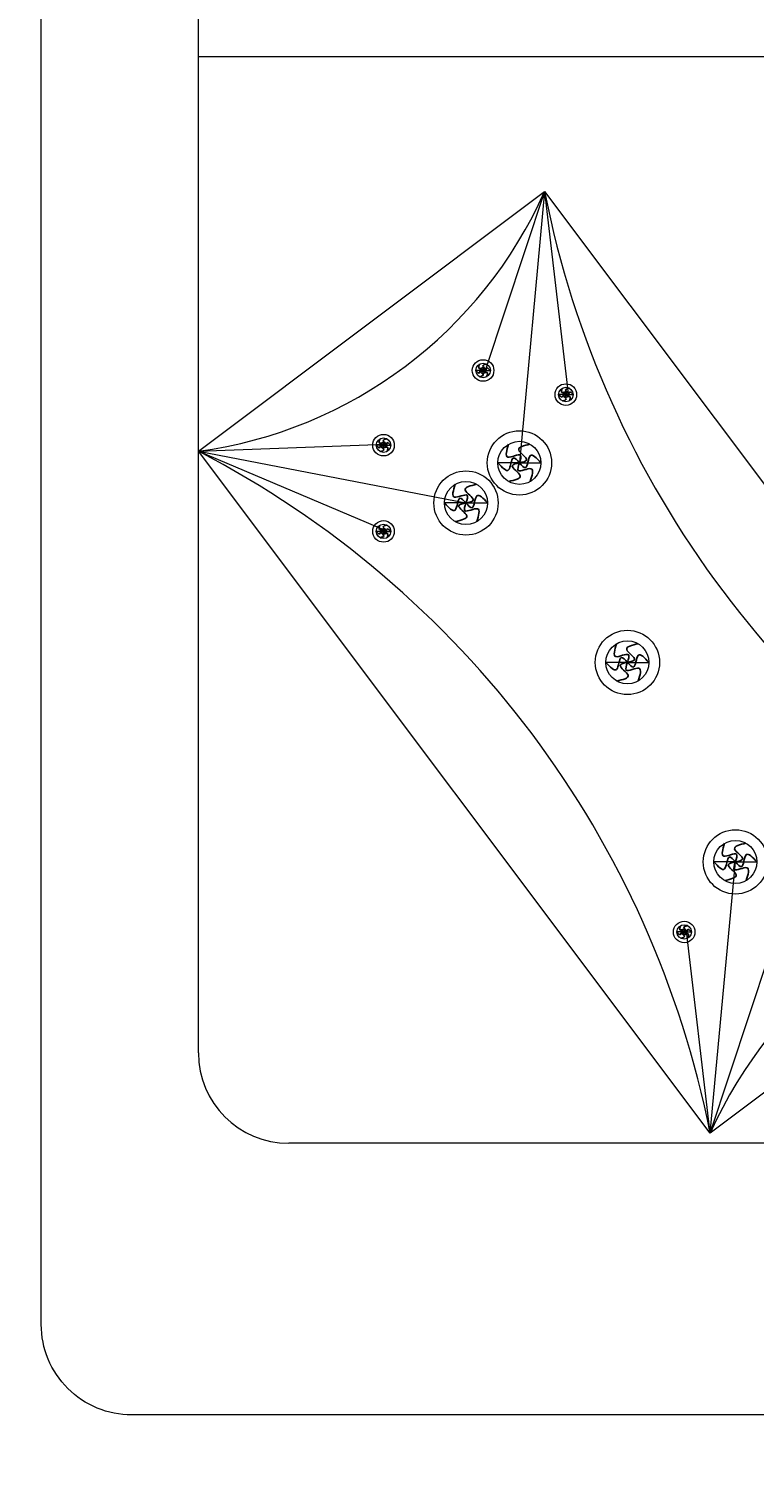
# Model space of a CAD drawing. Units: inches. Extents: x -61 to 1599, y -1316 to 257.
# Tile 102 of 204: x 126 to 142, y -131 to -99. Entities that reach past the tile are written whole.
import ezdxf

# ---------------------------------------------------------------- set-up
doc = ezdxf.new("R2010")
doc.units = ezdxf.units.IN
doc.header["$MEASUREMENT"] = 0
doc.layers.add('A-ANNO-DIMS', color=2, linetype='Continuous', lineweight=18)
doc.layers.add('FURNITURE', color=83, linetype='Continuous', lineweight=18)
doc.layers.add('FUR', color=83, linetype='Continuous')
doc.styles.get("Standard").update_dxf_attribs({"font": 'arial.ttf'})
doc.dimstyles.get("Standard").update_dxf_attribs({"dimtxt": 0.18, "dimasz": 0.18, "dimexe": 0.18, "dimexo": 0.0625, "dimgap": 0.09, "dimtad": 0, "dimtih": 1, "dimtoh": 1, "dimdec": 0, "dimzin": 0, "dimdsep": 46, "dimlunit": 3, "dimtxsty": 'Standard', "dimcen": 0.09, "dimadec": 0, "dimazin": 0, "dimtfac": 1, "dimtdec": 0, "dimtofl": 0, "dimtmove": 0, "dimatfit": 3, "dimfxl": 1, "dimtolj": 1, "dimtzin": 0, "dimarcsym": 0})

# ---------------------------------------------------------------- blocks, each defined once
blk = doc.blocks.new('*U160')
at = {"layer": 'FUR'}
blk.add_open_spline([(0.005, 0.08), (-0.03, 0.048), (-0.098, -0.015), (0.075, -0.018), (0.024, -0.063), (0.005, -0.08)], degree=3, knots=[0, 0, 0, 0, 0.0954578, 0.1898773, 0.2470677, 0.2470677, 0.2470677, 0.2470677], dxfattribs=at)
blk = doc.blocks.new('*U161')
at = {"layer": 'FUR', "transparency": 16777216}
for p, rotation in [((222.173, -79.977), 60), ((222.312, -79.968), 300), ((222.317, -80.048), 240), ((222.178, -80.056), 120), ((222.25, -80.092), 180)]:
    blk.add_blockref('*U160', p, dxfattribs=dict(at, rotation=rotation))
blk.add_blockref('*U160', (222.24, -79.932), dxfattribs=at)
blk = doc.blocks.new('*U172')
at = {"layer": 'FUR'}
blk.add_open_spline([(0.005, 0.08), (-0.03, 0.048), (-0.098, -0.015), (0.075, -0.018), (0.024, -0.063), (0.005, -0.08)], degree=3, knots=[0, 0, 0, 0, 0.0954578, 0.1898773, 0.2470677, 0.2470677, 0.2470677, 0.2470677], dxfattribs=at)
blk = doc.blocks.new('*U173')
at = {"layer": 'FUR', "transparency": 16777216}
for p, rotation in [((222.173, -79.977), 60), ((222.312, -79.968), 300), ((222.317, -80.048), 240), ((222.178, -80.056), 120), ((222.25, -80.092), 180)]:
    blk.add_blockref('*U172', p, dxfattribs=dict(at, rotation=rotation))
blk.add_blockref('*U172', (222.24, -79.932), dxfattribs=at)
blk = doc.blocks.new('*U184')
at = {"layer": 'FUR'}
blk.add_open_spline([(0.015, 0.238), (-0.088, 0.143), (-0.292, -0.045), (0.224, -0.053), (0.072, -0.187), (0.015, -0.238)], degree=3, knots=[0, 0, 0, 0, 0.2846533, 0.5662105, 0.736751, 0.736751, 0.736751, 0.736751], dxfattribs=at)
blk = doc.blocks.new('*U159')
at = {"layer": 'FUR', "transparency": 16777216}
for p, rotation in [((662.517, -238.489), 60), ((662.929, -238.463), 300), ((662.531, -238.727), 120), ((662.745, -238.833), 180), ((662.944, -238.702), 240)]:
    blk.add_blockref('*U184', p, dxfattribs=dict(at, rotation=rotation))
blk.add_blockref('*U184', (662.716, -238.357), dxfattribs=at)
blk = doc.blocks.new('*U174')
at = {"layer": 'FUR'}
blk.add_open_spline([(0.005, 0.08), (-0.03, 0.048), (-0.098, -0.015), (0.075, -0.018), (0.024, -0.063), (0.005, -0.08)], degree=3, knots=[0, 0, 0, 0, 0.0954578, 0.1898773, 0.2470677, 0.2470677, 0.2470677, 0.2470677], dxfattribs=at)
blk = doc.blocks.new('*U175')
at = {"layer": 'FUR', "transparency": 16777216}
for p, rotation in [((222.173, -79.977), 60), ((222.312, -79.968), 300), ((222.317, -80.048), 240), ((222.178, -80.056), 120), ((222.25, -80.092), 180)]:
    blk.add_blockref('*U174', p, dxfattribs=dict(at, rotation=rotation))
blk.add_blockref('*U174', (222.24, -79.932), dxfattribs=at)
blk = doc.blocks.new('*U168')
at = {"layer": 'FUR'}
blk.add_open_spline([(0.015, 0.238), (-0.088, 0.143), (-0.292, -0.045), (0.224, -0.053), (0.072, -0.187), (0.015, -0.238)], degree=3, knots=[0, 0, 0, 0, 0.2846533, 0.5662105, 0.736751, 0.736751, 0.736751, 0.736751], dxfattribs=at)
blk = doc.blocks.new('*U169')
at = {"layer": 'FUR', "transparency": 16777216}
for p, rotation in [((662.517, -238.489), 60), ((662.929, -238.463), 300), ((662.531, -238.727), 120), ((662.745, -238.833), 180), ((662.944, -238.702), 240)]:
    blk.add_blockref('*U168', p, dxfattribs=dict(at, rotation=rotation))
blk.add_blockref('*U168', (662.716, -238.357), dxfattribs=at)
blk = doc.blocks.new('*U176')
at = {"layer": 'FUR'}
blk.add_open_spline([(0.005, 0.08), (-0.03, 0.048), (-0.098, -0.015), (0.075, -0.018), (0.024, -0.063), (0.005, -0.08)], degree=3, knots=[0, 0, 0, 0, 0.0954578, 0.1898773, 0.2470677, 0.2470677, 0.2470677, 0.2470677], dxfattribs=at)
blk = doc.blocks.new('*U177')
at = {"layer": 'FUR', "transparency": 16777216}
for p, rotation in [((222.173, -79.977), 60), ((222.312, -79.968), 300), ((222.317, -80.048), 240), ((222.178, -80.056), 120), ((222.25, -80.092), 180)]:
    blk.add_blockref('*U176', p, dxfattribs=dict(at, rotation=rotation))
blk.add_blockref('*U176', (222.24, -79.932), dxfattribs=at)
blk = doc.blocks.new('*U170')
at = {"layer": 'FUR'}
blk.add_open_spline([(0.015, 0.238), (-0.088, 0.143), (-0.292, -0.045), (0.224, -0.053), (0.072, -0.187), (0.015, -0.238)], degree=3, knots=[0, 0, 0, 0, 0.2846533, 0.5662105, 0.736751, 0.736751, 0.736751, 0.736751], dxfattribs=at)
blk = doc.blocks.new('*U171')
at = {"layer": 'FUR', "transparency": 16777216}
for p, rotation in [((662.517, -238.489), 60), ((662.929, -238.463), 300), ((662.531, -238.727), 120), ((662.745, -238.833), 180), ((662.944, -238.702), 240)]:
    blk.add_blockref('*U170', p, dxfattribs=dict(at, rotation=rotation))
blk.add_blockref('*U170', (662.716, -238.357), dxfattribs=at)
blk = doc.blocks.new('*U164')
at = {"layer": 'FUR'}
blk.add_open_spline([(0.005, 0.08), (-0.03, 0.048), (-0.098, -0.015), (0.075, -0.018), (0.024, -0.063), (0.005, -0.08)], degree=3, knots=[0, 0, 0, 0, 0.0954578, 0.1898773, 0.2470677, 0.2470677, 0.2470677, 0.2470677], dxfattribs=at)
blk = doc.blocks.new('*U165')
at = {"layer": 'FUR', "transparency": 16777216}
for p, rotation in [((222.173, -79.977), 60), ((222.312, -79.968), 300), ((222.317, -80.048), 240), ((222.178, -80.056), 120), ((222.25, -80.092), 180)]:
    blk.add_blockref('*U164', p, dxfattribs=dict(at, rotation=rotation))
blk.add_blockref('*U164', (222.24, -79.932), dxfattribs=at)
blk = doc.blocks.new('*U183')
at = {"layer": 'FUR'}
blk.add_open_spline([(0.015, 0.238), (-0.088, 0.143), (-0.292, -0.045), (0.224, -0.053), (0.072, -0.187), (0.015, -0.238)], degree=3, knots=[0, 0, 0, 0, 0.2846533, 0.5662105, 0.736751, 0.736751, 0.736751, 0.736751], dxfattribs=at)
blk = doc.blocks.new('*U162')
at = {"layer": 'FUR', "transparency": 16777216}
for p, rotation in [((662.517, -238.489), 60), ((662.929, -238.463), 300), ((662.531, -238.727), 120), ((662.745, -238.833), 180), ((662.944, -238.702), 240)]:
    blk.add_blockref('*U183', p, dxfattribs=dict(at, rotation=rotation))
blk.add_blockref('*U183', (662.716, -238.357), dxfattribs=at)
blk = doc.blocks.new('SOFA-LOVESEAT')
for p, q in [((3.47, 8), (3.47, 52)), ((22.442, 30), (3.47, 30)), ((11.116, 27.026), (9.811, 23.092)), ((11.116, 27.026), (10.561, 21.032)), ((11.116, 27.026), (11.639, 22.56)), ((9.759, 23.073), (9.599, 23.073)), ((9.759, 23.073), (9.918, 23.073)), ((11.587, 22.541), (11.427, 22.541)), ((11.587, 22.541), (11.747, 22.541)), ((3.47, 21.288), (7.612, 21.442)), ((3.47, 21.288), (9.381, 20.146)), ((3.47, 21.288), (7.612, 19.538)), ((7.56, 21.423), (7.4, 21.423)), ((7.56, 21.423), (7.719, 21.423)), ((10.561, 21.032), (10.084, 21.032)), ((10.561, 21.032), (11.037, 21.032)), ((9.381, 20.146), (8.904, 20.146)), ((9.381, 20.146), (9.857, 20.146)), ((7.56, 19.518), (7.4, 19.518)), ((7.56, 19.518), (7.719, 19.518)), ((12.946, 16.624), (12.47, 16.624)), ((12.946, 16.624), (13.423, 16.624)), ((14.776, 6.223), (15.332, 12.217)), ((15.332, 12.217), (14.855, 12.217)), ((15.332, 12.217), (15.808, 12.217)), ((14.201, 10.669), (14.041, 10.669)), ((14.201, 10.669), (14.36, 10.669)), ((14.776, 6.223), (14.253, 10.689)), ((14.776, 6.223), (16.081, 10.156)), ((22.442, 6), (5.47, 6))]:
    blk.add_line(p, q)
blk.add_lwpolyline([(26, 6), (26, 2, -0.414214), (24, 0), (2, 0, -0.414214), (0, 2), (0, 58, -0.414213), (2, 60), (24, 60, -0.414214), (26, 58), (26, 54)], format="xyb")
blk.add_lwpolyline([(11.116, 27.026), (22.422, 11.961), (14.776, 6.223), (3.47, 21.288)], close=True)
for centre, radius in [((9.759, 23.073), 0.238), ((9.759, 23.073), 0.16), ((11.587, 22.541), 0.238), ((11.587, 22.541), 0.16), ((7.56, 21.423), 0.238), ((7.56, 21.423), 0.16), ((10.561, 21.032), 0.71), ((10.561, 21.032), 0.476), ((9.381, 20.146), 0.71), ((9.381, 20.146), 0.476), ((7.56, 19.518), 0.238), ((7.56, 19.518), 0.16), ((12.946, 16.624), 0.71), ((12.946, 16.624), 0.476), ((15.332, 12.217), 0.71), ((15.332, 12.217), 0.476), ((14.201, 10.669), 0.238), ((14.201, 10.669), 0.16)]:
    blk.add_circle(centre, radius)
for centre, radius, start, end in [((2.147, 31.014), 9.816, 277.747, 336.0258), ((32.433, 31.248), 21.731, 191.2044, 242.5684), ((-6.541, 2), 21.731, 11.2044, 62.5684), ((23.745, 2.234), 9.816, 97.747, 156.0258), ((5.47, 8), 2, 180, 270)]:
    blk.add_arc(centre, radius, start, end)
at = {"rotation": 90}
for name, p in [('*U175', (-70.254, -199.172)), ('*U177', (-68.425, -199.704)), ('*U173', (-72.453, -200.822)), ('*U169', (-228.034, -641.698)), ('*U159', (-229.214, -642.584)), ('*U161', (-72.453, -202.727)), ('*U171', (-225.649, -646.106)), ('*U162', (-223.264, -650.513)), ('*U165', (-65.812, -211.576))]:
    blk.add_blockref(name, p, dxfattribs=at)
blk = doc.blocks.new('*D687')
at = {"layer": 'A-ANNO-DIMS', "color": 0, "lineweight": -2, "transparency": 16777216}
for p, q in [((289.418, 181.677), (-61.077, 181.677)), ((-60.897, 181.497), (-60.897, -528.952)), ((-60.897, -1239.765), (-60.897, -529.316)), ((319.64, -1239.945), (-61.077, -1239.945))]:
    blk.add_line(p, q, dxfattribs=at)
at = {"layer": 'A-ANNO-DIMS', "color": 0, "transparency": 16777216}
for points in [[(-60.927, 181.497), (-60.867, 181.497), (-60.897, 181.677)], [(-60.927, -1239.765), (-60.867, -1239.765), (-60.897, -1239.945)]]:
    blk.add_solid(points, dxfattribs=at)
at = {"layer": 'DEFPOINTS', "color": 0, "transparency": 16777216}
for p in [(289.481, 181.677), (-60.897, -1239.945), (319.703, -1239.945)]:
    blk.add_point(p, dxfattribs=at)
at = {"layer": 'A-ANNO-DIMS', "color": 0, "transparency": 16777216, "insert": (-60.897, -529.134), "char_height": 0.18, "attachment_point": 5}
blk.add_mtext('\\A1;1421.6', dxfattribs=at)
blk = doc.blocks.new('*D700')
at = {"layer": 'A-ANNO-DIMS', "color": 0, "lineweight": -2, "transparency": 16777216}
for p, q in [((14.703, -616.882), (14.703, 257.457)), ((179.752, -616.882), (179.752, 257.457)), ((14.883, 257.277), (96.772, 257.277)), ((179.572, 257.277), (97.683, 257.277))]:
    blk.add_line(p, q, dxfattribs=at)
at = {"layer": 'A-ANNO-DIMS', "color": 0, "transparency": 16777216}
for points in [[(14.883, 257.307), (14.883, 257.247), (14.703, 257.277)], [(179.572, 257.307), (179.572, 257.247), (179.752, 257.277)]]:
    blk.add_solid(points, dxfattribs=at)
at = {"layer": 'DEFPOINTS', "color": 0, "transparency": 16777216}
for p in [(179.752, 257.277), (14.703, -616.945), (179.752, -616.945)]:
    blk.add_point(p, dxfattribs=at)
at = {"layer": 'A-ANNO-DIMS', "color": 0, "transparency": 16777216, "insert": (97.227, 257.277), "char_height": 0.18, "attachment_point": 5}
blk.add_mtext('\\A1;165.05', dxfattribs=at)

msp = doc.modelspace()

# ---------------------------------------------------------------- block references
at = {"layer": 'FURNITURE'}
msp.add_blockref('SOFA-LOVESEAT', (125.901, -129.695), dxfattribs=at)

# ---------------------------------------------------------------- dimensions: what is measured, and where the dimension line sits
at = {"layer": 'A-ANNO-DIMS'}
dim = msp.add_linear_dim(base=(179.7521, 257.2771), p1=(14.7028, -616.9446), p2=(179.7521, -616.9446), dimstyle='Standard', override={"dimdec": 2, "dimlfac": 1, "dimrnd": 0, "dimzin": 0, "dimdsep": 46, "dimlunit": 2}, dxfattribs=at)
dim.commit()
dim.dimension.update_dxf_attribs({"geometry": '*D700', "text_midpoint": (97.2274, 257.2771)})
dim = msp.add_linear_dim(base=(-60.8972, -1239.9446), p1=(289.4807, 181.6771), p2=(319.7028, -1239.9446), angle=90, dimstyle='Standard', override={"dimdec": 1, "dimlfac": 1, "dimrnd": 0, "dimzin": 0, "dimdsep": 46, "dimlunit": 2}, dxfattribs=at)
dim.commit()
dim.dimension.update_dxf_attribs({"geometry": '*D687', "text_midpoint": (-60.8972, -529.1337)})

doc.saveas('drawing.dxf')
